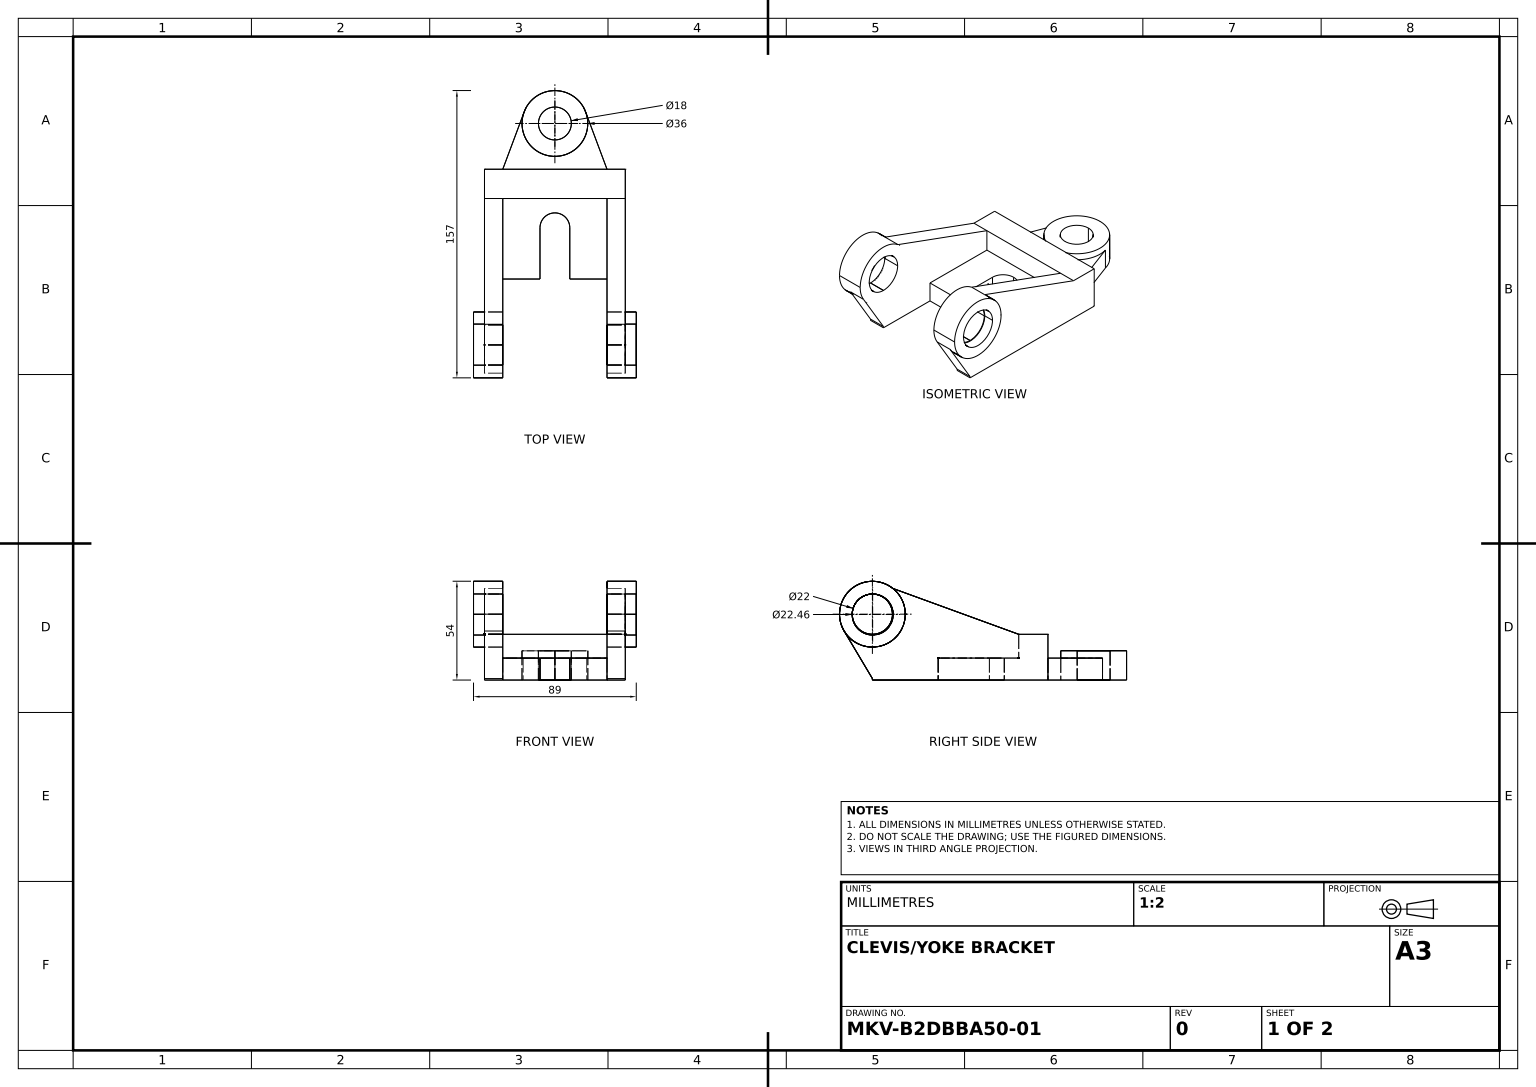
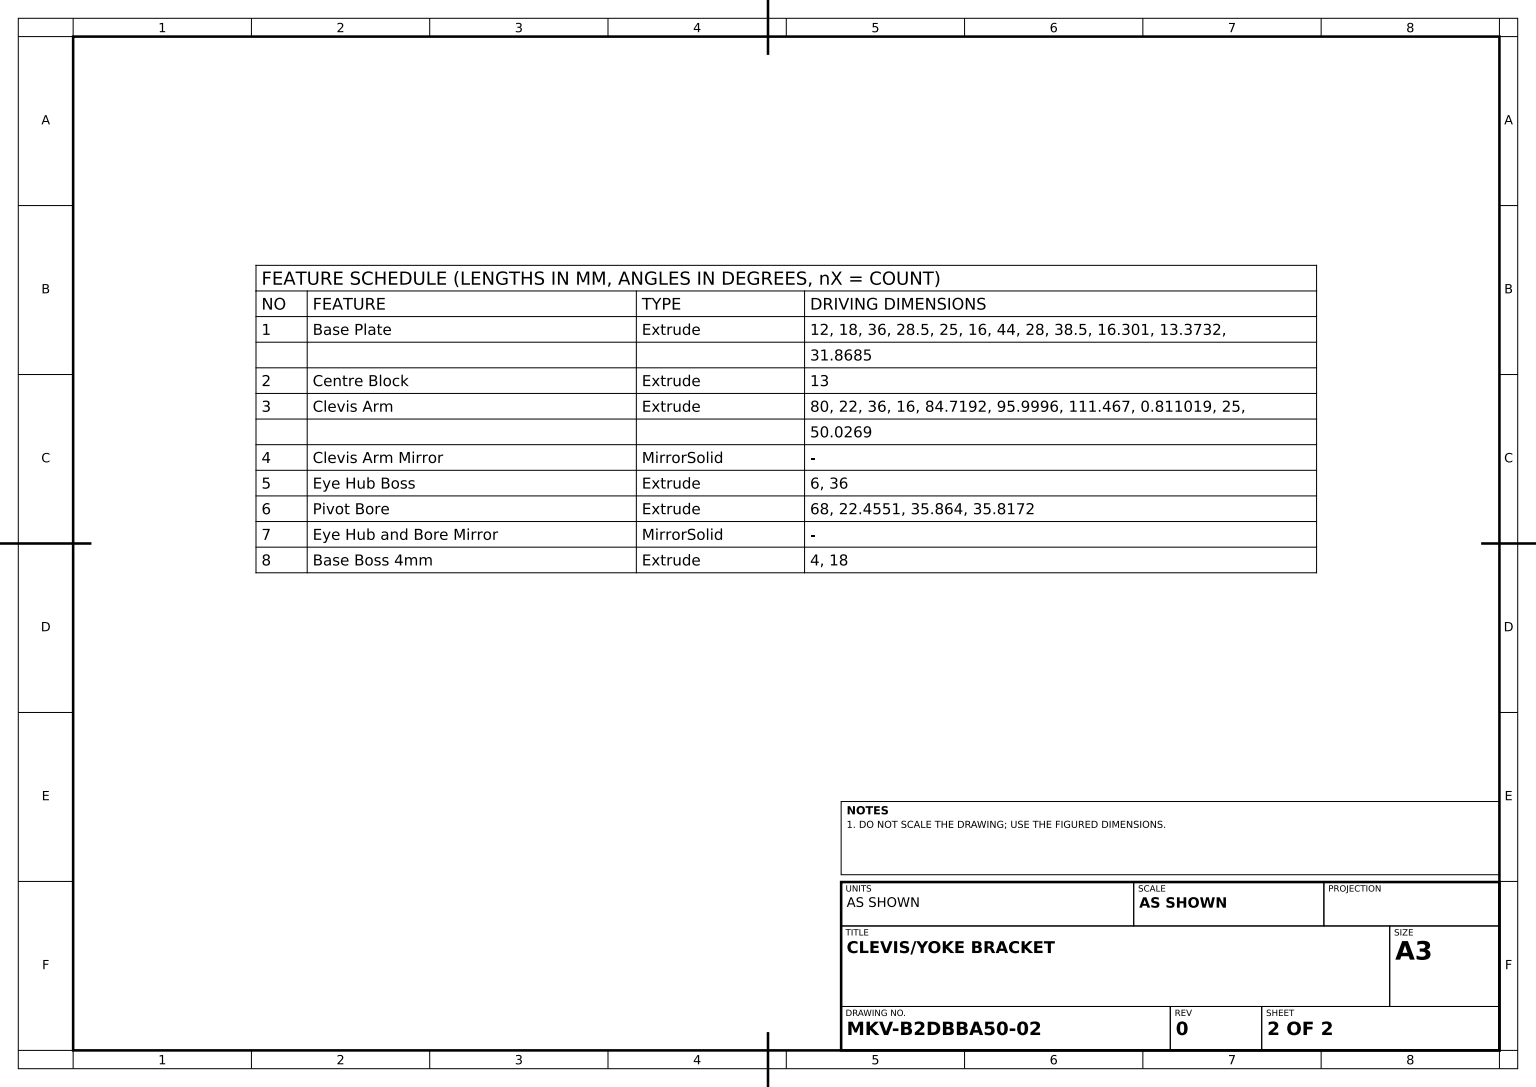
from build123d import *

# Parameters (mm, degrees)
BASE_PLATE_SKETCH_R   = 18
BASE_PLATE_SKETCH_R_2 = 9
BASE_PLATE_DEPTH      = 12
CENTRE_BLOCK_SKETCH_W = 77
CENTRE_BLOCK_SKETCH_H = 16
CENTRE_BLOCK_DEPTH    = 13
CLEVIS_ARM_DEPTH      = 10
EYE_HUB_SKETCH_R      = 18
EYE_HUB_BOSS_DEPTH    = 6
PIVOT_BORE_SKETCH_R   = 11.227532681
PIVOT_BORE_DEPTH      = 68
BASE_BOSS_SKETCH_R    = 18
BASE_BOSS_SKETCH_R_2  = 9
BASE_BOSS_4MM_DEPTH   = 4


with BuildPart() as part:
    # Base Plate Sketch → Base Plate (new body)
    # profile 1 of 4: a face of its own
    with BuildSketch(Plane(origin=(0, 0, 0), x_dir=(1, 0, 0), z_dir=(0, 1, 0))):
        with BuildLine():
            ThreePointArc((8.150523058, -45.373183795), (0, -37.222660737), (-8.150523058, -45.373183795))
            Line((-8.150523058, -45.373183795), (-8.150523058, -73.373183795))
            Line((-8.150523058, -73.373183795), (-28.5, -73.373183795))
            Line((-28.5, -73.373183795), (-28.5, -29.373183795))
            Line((-28.5, -29.373183795), (28.5, -29.373183795))
            Line((28.5, -29.373183795), (28.5, -73.373183795))
            Line((28.5, -73.373183795), (8.150523058, -73.373183795))
            Line((8.150523058, -73.373183795), (8.150523058, -45.373183795))
        make_face()
    # profile 2 of 4: a face of its own
    with BuildSketch(Plane(origin=(0, 0, 0), x_dir=(1, 0, 0), z_dir=(0, 1, 0))):
        Polygon((28.5, -13.373183795), (0, -13.373183795), (-28.5, -13.373183795), (-38.5, -13.373183795), (-38.5, -29.373183795), (-28.5, -29.373183795), (28.5, -29.373183795), (38.5, -29.373183795), (38.5, -13.373183795), align=None)
    # profile 3 of 4: a face of its own
    with BuildSketch(Plane(origin=(0, 0, 0), x_dir=(1, 0, 0), z_dir=(0, 1, 0))):
        with BuildLine():
            Line((-28.5, -13.373183795), (0, -13.373183795))
            Line((0, -13.373183795), (28.5, -13.373183795))
            Line((28.5, -13.373183795), (17.334695629, 16.475354899))
            ThreePointArc((17.334695629, 16.475354899), (17.832898269, 14.073801972), (18, 11.626816205))
            ThreePointArc((18, 11.626816205), (-2.446985767, -6.206082063), (-17.334695629, 16.475354899))
            Line((-17.334695629, 16.475354899), (-28.5, -13.373183795))
        make_face()
    # profile 4 of 4: a face of its own
    with BuildSketch(Plane(origin=(0, 0, 0), x_dir=(1, 0, 0), z_dir=(0, 1, 0))):
        with Locations((0, 11.626816205)):
            Circle(BASE_PLATE_SKETCH_R)
        with Locations(Location((0, 11.626816205, 0), (0, 0, 270))):
            Circle(BASE_PLATE_SKETCH_R_2, mode=Mode.SUBTRACT)
    extrude(amount=BASE_PLATE_DEPTH)

    # Centre Block Sketch → Centre Block (add)
    with BuildSketch(Plane(origin=(0, 12, 0), x_dir=(1, 0, 0), z_dir=(0, 1, 0))):
        with Locations((0, -21.373183795)):
            Rectangle(CENTRE_BLOCK_SKETCH_W, CENTRE_BLOCK_SKETCH_H)
    extrude(amount=CENTRE_BLOCK_DEPTH)

    # Clevis Arm Sketch → Clevis Arm (add)
    # profile 1 of 2: a face of its own
    with BuildSketch(Plane(origin=(38.5, 0, 0), x_dir=(0, 0, -1), z_dir=(1, 0, 0))):
        with BuildLine():
            Line((-29.373183795, 0), (-29.373183795, 24.999999998))
            Line((-29.373183795, 24.999999998), (-98.092419727, 50.026895655))
            ThreePointArc((-98.092419726, 50.026895656), (-93.139370455, 43.776688822), (-91.372765384, 35.999999998))
            ThreePointArc((-91.372765384, 35.999999998), (-104.59810148, 18.644811016), (-124.839719228, 26.792756176))
            Line((-124.839719228, 26.792756176), (-109.373183795, 0.811018934))
            Line((-109.373183795, 0.811018934), (-109.373183795, 0))
            Line((-109.373183795, 0), (-29.373183795, 0))
        make_face()
    # profile 2 of 2: a face of its own
    with BuildSketch(Plane(origin=(38.5, 0, 0), x_dir=(0, 0, -1), z_dir=(1, 0, 0))):
        with BuildLine():
            ThreePointArc((-91.372765384, 35.999999998), (-93.139370455, 43.776688822), (-98.092419726, 50.026895656))
            ThreePointArc((-98.092419726, 50.026895656), (-121.176926997, 49.589031186), (-124.839719228, 26.792756176))
            ThreePointArc((-124.839719228, 26.792756176), (-104.59810148, 18.644811016), (-91.372765384, 35.999999998))
        make_face()
        with BuildLine():
            ThreePointArc((-98.372765384, 35.999999998), (-101.594590791, 28.221825405), (-109.372765384, 24.999999998))
            Line((-109.372765384, 24.999999998), (-109.373183795, 24.999999998))
            ThreePointArc((-109.373183795, 25.000000006), (-117.150792046, 43.77832252), (-98.372765384, 35.999999998))
        make_face(mode=Mode.SUBTRACT)
    extrude(amount=-CLEVIS_ARM_DEPTH)

    # Clevis Arm Mirror: part across plane


with BuildPart() as part_1:
    add(part.part)
    add(part.part.mirror(Plane(origin=(0, 0, 0), x_dir=(0, 0, 1), z_dir=(1, 0, 0))))

    # Eye Hub Sketch → Eye Hub Boss (add)
    with BuildSketch(Plane(origin=(38.5, 0, 0), x_dir=(0, 0, -1), z_dir=(1, 0, 0))):
        with Locations((-109.372765384, 35.999999998)):
            Circle(EYE_HUB_SKETCH_R)
    extrude(amount=EYE_HUB_BOSS_DEPTH)

    # Pivot Bore Sketch → Pivot Bore (cut)
    with BuildSketch(Plane.ZY.offset(-28.5)):
        with Locations((109.237217655, 35.817248986)):
            Circle(PIVOT_BORE_SKETCH_R)
    extrude(amount=-PIVOT_BORE_DEPTH, mode=Mode.SUBTRACT)

    # Eye Hub and Bore Mirror: part across plane


with BuildPart() as part_2:
    add(part_1.part)
    add(part_1.part.mirror(Plane(origin=(0, 0, 0), x_dir=(0, 0, 1), z_dir=(1, 0, 0))))

    # Base Boss Sketch → Base Boss 4mm (add)
    with BuildSketch(Plane(origin=(0, 12, 0), x_dir=(1, 0, 0), z_dir=(0, 1, 0))):
        with Locations(Location((0, 11.626816205, 0), (0, 0, 164.373619322))):
            Circle(BASE_BOSS_SKETCH_R)
        with Locations(Location((0, 11.626816205, 0), (0, 0, 270))):
            Circle(BASE_BOSS_SKETCH_R_2, mode=Mode.SUBTRACT)
    extrude(amount=BASE_BOSS_4MM_DEPTH)


solid = part_2.part
